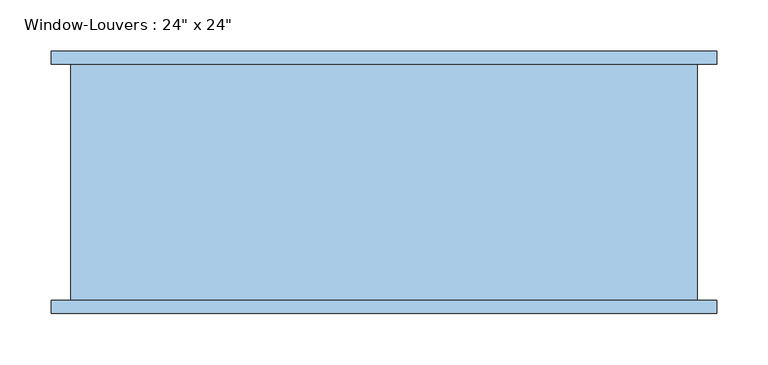
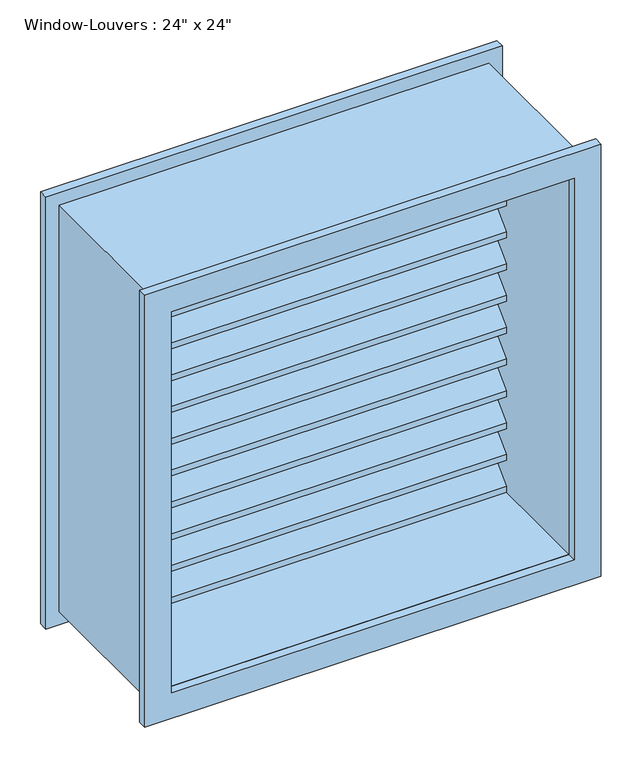
"""IFC4 building model written with IfcOpenShell, lengths in millimetres: window geometry."""

from ifc_helpers import new_model, si_unit, frame, origin, place, context, project, spatial, polyline, outline, extrude, source, transform, mapped, element, save


def window_6da96920(model_context):
    return source(origin(), model_context, "Body", "SweptSolid", [
        extrude(outline(polyline([(108.65, 1419.1754778), (108.65, 1410.1952217), (70.55, 1448.2952217), (32.45, 1410.1952217), (32.45, 1419.1754778), (70.55, 1457.2754778), (108.65, 1419.1754778)])), frame((-285.75, 0.0, 0.0), z_axis=(1.0, 0.0, 0.0), x_axis=(0.0, 1.0, 0.0)), (0.0, 0.0, 1.0), 571.5),
        extrude(outline(polyline([(108.65, 1371.5009557), (108.65, 1362.5206995), (70.55, 1400.6206995), (32.45, 1362.5206995), (32.45, 1371.5009557), (70.55, 1409.6009557), (108.65, 1371.5009557)])), frame((-285.75, 0.0, 0.0), z_axis=(1.0, 0.0, 0.0), x_axis=(0.0, 1.0, 0.0)), (0.0, 0.0, 1.0), 571.5),
        extrude(outline(polyline([(108.65, 1323.8264335), (108.65, 1314.8461774), (70.55, 1352.9461774), (32.45, 1314.8461774), (32.45, 1323.8264335), (70.55, 1361.9264335), (108.65, 1323.8264335)])), frame((-285.75, 0.0, 0.0), z_axis=(1.0, 0.0, 0.0), x_axis=(0.0, 1.0, 0.0)), (0.0, 0.0, 1.0), 571.5),
        extrude(outline(polyline([(108.65, 1276.1519113), (108.65, 1267.1716552), (70.55, 1305.2716552), (32.45, 1267.1716552), (32.45, 1276.1519113), (70.55, 1314.2519113), (108.65, 1276.1519113)])), frame((-285.75, 0.0, 0.0), z_axis=(1.0, 0.0, 0.0), x_axis=(0.0, 1.0, 0.0)), (0.0, 0.0, 1.0), 571.5),
        extrude(outline(polyline([(108.65, 1228.4773891), (108.65, 1219.497133), (70.55, 1257.597133), (32.45, 1219.497133), (32.45, 1228.4773891), (70.55, 1266.5773891), (108.65, 1228.4773891)])), frame((-285.75, 0.0, 0.0), z_axis=(1.0, 0.0, 0.0), x_axis=(0.0, 1.0, 0.0)), (0.0, 0.0, 1.0), 571.5),
        extrude(outline(polyline([(108.65, 1180.802867), (108.65, 1171.8226109), (70.55, 1209.9226109), (32.45, 1171.8226109), (32.45, 1180.802867), (70.55, 1218.902867), (108.65, 1180.802867)])), frame((-285.75, 0.0, 0.0), z_axis=(1.0, 0.0, 0.0), x_axis=(0.0, 1.0, 0.0)), (0.0, 0.0, 1.0), 571.5),
        extrude(outline(polyline([(108.65, 1133.1283448), (108.65, 1124.1480887), (70.55, 1162.2480887), (32.45, 1124.1480887), (32.45, 1133.1283448), (70.55, 1171.2283448), (108.65, 1133.1283448)])), frame((-285.75, 0.0, 0.0), z_axis=(1.0, 0.0, 0.0), x_axis=(0.0, 1.0, 0.0)), (0.0, 0.0, 1.0), 571.5),
        extrude(outline(polyline([(108.65, 1085.4538226), (108.65, 1076.4735665), (70.55, 1114.5735665), (32.45, 1076.4735665), (32.45, 1085.4538226), (70.55, 1123.5538226), (108.65, 1085.4538226)])), frame((-285.75, 0.0, 0.0), z_axis=(1.0, 0.0, 0.0), x_axis=(0.0, 1.0, 0.0)), (0.0, 0.0, 1.0), 571.5),
        extrude(outline(polyline([(108.65, 1037.7793005), (108.65, 1028.7990443), (70.55, 1066.8990443), (32.45, 1028.7990443), (32.45, 1037.7793005), (70.55, 1075.8793005), (108.65, 1037.7793005)])), frame((-285.75, 0.0, 0.0), z_axis=(1.0, 0.0, 0.0), x_axis=(0.0, 1.0, 0.0)), (0.0, 0.0, 1.0), 571.5),
        extrude(outline(polyline([(108.65, 990.1047783), (108.65, 981.1245222), (70.55, 1019.2245222), (32.45, 981.1245222), (32.45, 990.1047783), (70.55, 1028.2047783), (108.65, 990.1047783)])), frame((-285.75, 0.0, 0.0), z_axis=(1.0, 0.0, 0.0), x_axis=(0.0, 1.0, 0.0)), (0.0, 0.0, 1.0), 571.5),
        extrude(outline(polyline([(108.65, 1466.85), (108.65, 1457.8697439), (70.55, 1495.9697439), (32.45, 1457.8697439), (32.45, 1466.85), (70.55, 1504.95), (108.65, 1466.85)])), frame((-285.75, 0.0, 0.0), z_axis=(1.0, 0.0, 0.0), x_axis=(0.0, 1.0, 0.0)), (0.0, 0.0, 1.0), 571.5),
        extrude(outline(polyline([(108.65, 942.4302561), (108.65, 933.45), (70.55, 971.55), (32.45, 933.45), (32.45, 942.4302561), (70.55, 980.5302561), (108.65, 942.4302561)])), frame((-285.75, 0.0, 0.0), z_axis=(1.0, 0.0, 0.0), x_axis=(0.0, 1.0, 0.0)), (0.0, 0.0, 1.0), 571.5),
        extrude(outline(polyline([(1524.0, 304.8), (1524.0, -304.8), (914.4, -304.8), (914.4, 304.8), (1524.0, 304.8)]), holes=[polyline([(1504.95, 285.75), (933.45, 285.75), (933.45, -285.75), (1504.95, -285.75), (1504.95, 285.75)])]), frame((0.0, -121.35, 0.0), z_axis=(0.0, 1.0, 0.0), x_axis=(0.0, 0.0, 1.0)), (0.0, 0.0, 1.0), 230.0),
        extrude(outline(polyline([(1543.05, 323.85), (1543.05, -323.85), (895.35, -323.85), (895.35, 323.85), (1543.05, 323.85)]), holes=[polyline([(1504.95, 285.75), (933.45, 285.75), (933.45, -285.75), (1504.95, -285.75), (1504.95, 285.75)])]), frame((0.0, -134.05, 0.0), z_axis=(0.0, 1.0, 0.0), x_axis=(0.0, 0.0, 1.0)), (0.0, 0.0, 1.0), 12.7),
        extrude(outline(polyline([(1543.05, -323.85), (895.35, -323.85), (895.35, 323.85), (1543.05, 323.85), (1543.05, -323.85)]), holes=[polyline([(1504.95, -285.75), (1504.95, 285.75), (933.45, 285.75), (933.45, -285.75), (1504.95, -285.75)])]), frame((0.0, 108.65, 0.0), z_axis=(0.0, 1.0, 0.0), x_axis=(0.0, 0.0, 1.0)), (0.0, 0.0, 1.0), 12.7),
    ])


if __name__ == "__main__":
    model = new_model("IFC4")
    model_context = context("Model", 3, world=origin())
    ifc_project = project(units=[si_unit("LENGTHUNIT", "METRE", prefix="MILLI")], contexts=[model_context])
    site = spatial("IfcSite", under=ifc_project)
    building = spatial("IfcBuilding", under=site)
    placement = place(None, origin())
    window_shape = window_6da96920(model_context)
    element("IfcWindow", 1, ObjectType="Window-Louvers : 24\" x 24\"", at=placement, inside=building, context=model_context, shape_type="MappedRepresentation", body=[
        mapped(window_shape, transform((0.0, 0.0, 0.0), x_axis=(1.0, 0.0, 0.0), y_axis=(0.0, 1.0, 0.0), z_axis=(0.0, 0.0, 1.0))),
    ])
    save(model, "model.ifc")

# Revit data of these elements
# Type "Window-Louvers : 24\" x 24\""
#   Type Mark = "V"
#   Construction Type Id = "GSP4R"
#   Assembly Code = "B20"
#   Analytic Construction = "1/8 in Pilkington single glazing"
#   Visual Light Transmittance = 0.9
#   Thermal Resistance (R) = 1.53941 (h·ft²·°F)/BTU
#   Solar Heat Gain Coefficient = 0.78
#   Max Height = 1' - 11.74264"
#   Height = 2' - 0"
#   Heat Transfer Coefficient (U) = 0.6496 BTU/(h·ft²·°F)
#   Blade Width [instance default] = 1' - 10 1/2"
#   Blade Vertical Thickness = 0' - 0.35355"
#   Blade Thickness = 0' - 0 1/4"
#   Blade Spacing = 0' - 1 1/2"
#   Blade Height = 0' - 1.85355"
#   Blade Depth = 0' - 3"
#   Blade Angle = 45.00°
#   Default Sill Height = 3' - 0"
#   Trim Projection_Exterior = 0' - 0 1/2"
#   Trim Projection_Interior = 0' - 0 1/2"
#   Trim Width_Exterior = 0' - 1 1/2"
#   Trim Width_Interior = 0' - 1 1/2"
#   Width = 2' - 0"
#   Max Blade Count = 12
#   Define Thermal Properties by = 1
#   Blade Count = 12
#   Frame Material = Birch
#   Louver Material = Birch
#   Trim Exterior Material = Birch
#   Trim Interior Material = Birch
#   Wall Closure = (empty or 0)
# Element 1 (IfcWindow, "Window-Louvers : 24\" x 24\"")
#   Materials on its faces: "Birch"
# Materials
#   "Birch": class "Wood", colour RGB 224 178 126, transparency 0, Description = "Betula Alleghaniensis", Cost = 0
